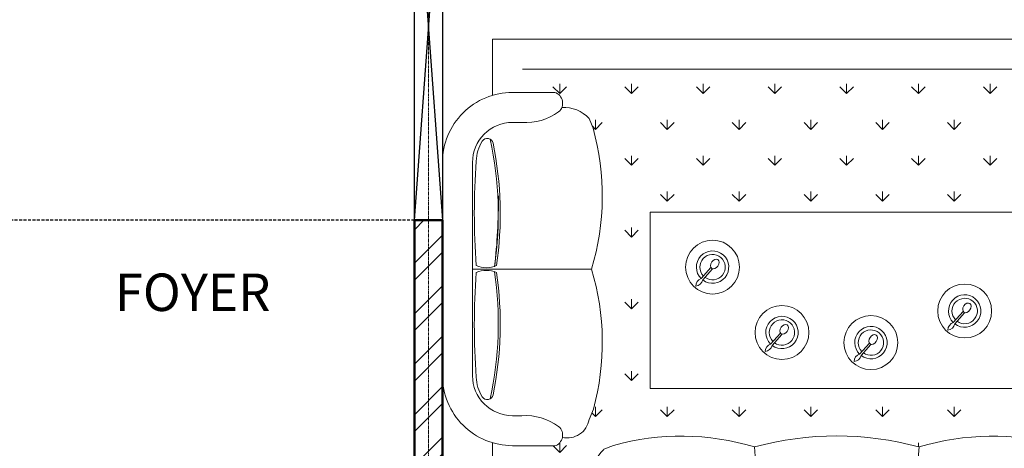
# Model space of a CAD drawing. Units: inches. Extents: x 261 to 2725, y 291 to 1454.
# Tile 10 of 35: x 688 to 898, y 550 to 641. Entities that reach past the tile are written whole.
import ezdxf

# ---------------------------------------------------------------- set-up
doc = ezdxf.new("R2010")
doc.units = ezdxf.units.IN
doc.linetypes.add('CENTER', pattern=[2, 1.25, -0.25, 0.25, -0.25])
doc.linetypes.add('DASHED', pattern=[19.05, 12.7, -6.35])
for name, color, linetype, lineweight in [('A-ANNO-DIMS', 136, 'Continuous', 18), ('A-AREA-IDEN', 18, 'Continuous', 18), ('A-FURN', 30, 'Continuous', 18), ('A-GRID', 251, 'CENTER', 13), ('A-ROOF-PRGL', 25, 'Continuous', 25), ('A-WALL', 222, 'Continuous', 50), ('A-WALL-OVHD', 222, 'DASHED', 25), ('A-WALL-PATT', 243, 'Continuous', 13)]:
    doc.layers.add(name, color=color, linetype=linetype, lineweight=lineweight)
doc.styles.get("Standard").update_dxf_attribs({"font": 'arial.ttf'})
doc.dimstyles.new('ISO-25', dxfattribs={"dimtxt": 12, "dimasz": 6, "dimexe": 1.25, "dimexo": 0.625, "dimtad": 1, "dimdec": 0, "dimlunit": 3, "dimtxsty": 'Standard', "dimblk": 'ARCHTICK', "dimcen": 2.5, "dimadec": 0, "dimazin": 0, "dimtfac": 1, "dimtdec": 0, "dimtmove": 0, "dimatfit": 3, "dimfxl": 1, "dimfxlon": 1, "dimarcsym": 0})

# ---------------------------------------------------------------- blocks, each defined once
blk = doc.blocks.new('A$C29956593')
for p, q in [((1017.8, 2786), (2742.6, 2786)), ((2910.7, 2786), (2742.6, 2786)), ((3602, 2800.7), (3586.8, 2719.3)), ((3630, 2728.1), (3602, 2800.7)), ((3742.2, 2770.6), (3716.5, 2736.8)), ((3730.5, 2659.2), (3742.2, 2770.6)), ((303.3, 2712.1), (296.9, 2710.1)), ((306.1, 2701.8), (303.3, 2712.1)), ((869.5, 2753), (870.7, 2751.8)), ((3447.8, 2749.3), (3463, 2718.1)), ((3486.3, 2729.3), (3447.8, 2749.3)), ((3463, 2718.1), (3488.7, 2658)), ((3547.1, 2656.7), (3486.3, 2729.3)), ((3551.8, 2734.3), (3547.1, 2656.7)), ((3586.8, 2684.2), (3551.8, 2734.3)), ((3586.8, 2719.3), (3589.1, 2643)), ((3644.1, 2670.5), (3630, 2728.1)), ((3716.5, 2736.8), (3682.6, 2663)), ((3811.1, 2721.8), (3772.6, 2710.5)), ((3792.4, 2665.5), (3811.1, 2721.8)), ((113, 2666.3), (113, 2216.3)), ((563, 2666.3), (113, 2666.3)), ((257.1, 2665), (256.2, 2657.4)), ((265.8, 2668.1), (257.1, 2665)), ((259.7, 2679.5), (257.9, 2671.6)), ((257.9, 2671.6), (265.8, 2668.1)), ((269.9, 2678.1), (259.7, 2679.5)), ((268, 2691.2), (264.2, 2685.9)), ((264.2, 2685.9), (269.9, 2678.1)), ((267.7, 2639.4), (270.2, 2671)), ((276.9, 2686.9), (268, 2691.2)), ((270.2, 2671), (283.9, 2691.1)), ((278.2, 2702.6), (273.3, 2697.8)), ((273.3, 2697.8), (276.9, 2686.9)), ((285.5, 2696.3), (278.2, 2702.6)), ((283.9, 2691.1), (302.3, 2697.9)), ((290.3, 2707.8), (284.9, 2706)), ((284.9, 2706), (285.5, 2696.3)), ((296.9, 2700.7), (290.3, 2707.8)), ((296.9, 2710.1), (296.9, 2700.7)), ((302.3, 2697.9), (322.4, 2697.8)), ((309.1, 2711), (306.1, 2701.8)), ((314.8, 2711.2), (309.1, 2711)), ((318.9, 2702.4), (314.8, 2711.2)), ((322.6, 2710.2), (318.9, 2702.4)), ((322.4, 2697.8), (339.2, 2688.6)), ((328.8, 2709.2), (322.6, 2710.2)), ((327.9, 2698.5), (328.8, 2709.2)), ((333.7, 2706), (327.9, 2698.5)), ((338.4, 2703.2), (333.7, 2706)), ((338.4, 2693.8), (338.4, 2703.2)), ((345.6, 2700), (338.4, 2693.8)), ((339.2, 2688.6), (351, 2673.6)), ((351, 2695.6), (345.6, 2700)), ((345.9, 2686.3), (351, 2695.6)), ((355.4, 2689.1), (345.9, 2686.3)), ((351, 2673.6), (355.9, 2654.7)), ((354.8, 2675.8), (359.4, 2683.1)), ((363.7, 2677.8), (354.8, 2675.8)), ((359.4, 2683.1), (355.4, 2689.1)), ((358, 2664.3), (365.7, 2670.6)), ((367.5, 2662.1), (358, 2664.3)), ((365.7, 2670.6), (363.7, 2677.8)), ((563, 2216.3), (563, 2666.3)), ((3395.2, 2706.8), (3416.2, 2674.3)), ((3453.6, 2676.8), (3395.2, 2706.8)), ((3416.2, 2674.3), (3463, 2616.7)), ((3502.7, 2650.5), (3453.6, 2676.8)), ((3682.6, 2663), (3610.3, 2495.9)), ((3635.9, 2584.1), (3644.1, 2670.5)), ((3772.6, 2710.5), (3732.8, 2670.5)), ((3766.7, 2622.9), (3792.4, 2665.5)), ((255.7, 2654.1), (254.5, 2644.2)), ((254.5, 2644.2), (263.6, 2641.2)), ((263.6, 2641.2), (254.7, 2635.1)), ((254.7, 2635.1), (255.8, 2629)), ((265.6, 2653.6), (255.7, 2654.1)), ((255.8, 2629), (265, 2627.7)), ((256.2, 2657.4), (265.6, 2653.6)), ((265, 2627.7), (257.1, 2621.8)), ((257.1, 2621.8), (257.6, 2614.3)), ((257.6, 2614.3), (266.7, 2613.4)), ((266.7, 2613.4), (258.5, 2609)), ((269.6, 2618.4), (267.7, 2639.4)), ((267.7, 2616.4), (269.6, 2618.4)), ((269.4, 2615), (267.7, 2616.4)), ((270.3, 2600.3), (269.4, 2615)), ((345.1, 2616), (342.8, 2608.6)), ((349.3, 2635.7), (345.1, 2629.6)), ((345.1, 2629.6), (348.7, 2623.5)), ((348.7, 2623.5), (345.1, 2616)), ((346.5, 2598), (349, 2613.2)), ((349, 2613.2), (352.7, 2620.7)), ((355.9, 2654.7), (349.3, 2635.7)), ((352.6, 2622.8), (357.2, 2624.6)), ((352.7, 2620.7), (352.6, 2622.8)), ((353.1, 2636.5), (363.4, 2637.8)), ((360.9, 2631.3), (353.1, 2636.5)), ((357.2, 2624.6), (360.9, 2631.3)), ((357.4, 2651), (368.4, 2653.8)), ((366.3, 2646), (357.4, 2651)), ((363.4, 2637.8), (366.3, 2646)), ((368.4, 2653.8), (367.5, 2662.1)), ((2910.7, 2636), (1017.8, 2636)), ((1552.3, 2040.1), (1598.4, 2636)), ((2376.2, 2040.1), (2336.4, 2636)), ((3463, 2616.7), (3512, 2567.8)), ((3557.6, 2604.2), (3502.7, 2650.5)), ((3545.9, 2656.7), (3559.9, 2601.7)), ((3589.1, 2643), (3606.7, 2581.6)), ((3686.1, 2581.6), (3730.5, 2659.2)), ((3727.7, 2578), (3766.7, 2622.9)), ((3859, 2620.4), (3783.1, 2611.7)), ((3891.7, 2610.4), (3859, 2620.4)), ((216.6, 2403), (304.3, 2601.6)), ((231.9, 2406.6), (308.2, 2579.2)), ((258.5, 2609), (258.5, 2601.3)), ((258.5, 2601.3), (267.9, 2601.3)), ((267.9, 2601.3), (258.9, 2597.3)), ((258.9, 2597.3), (259.1, 2591.7)), ((259.1, 2591.7), (268.7, 2590.5)), ((268.7, 2590.5), (260.3, 2584.2)), ((260.3, 2584.2), (260.7, 2578.8)), ((260.7, 2578.8), (269.3, 2577.7)), ((261.3, 2572.2), (261.1, 2568.5)), ((261.1, 2568.5), (263.9, 2566.2)), ((269.3, 2577.7), (261.3, 2572.2)), ((263.9, 2566.2), (269, 2563.6)), ((269.2, 2568), (274, 2569.4)), ((272.1, 2566.8), (269.2, 2568)), ((272.6, 2580.5), (270.3, 2600.3)), ((273.1, 2564.2), (272.1, 2566.8)), ((274, 2569.4), (272.6, 2580.5)), ((275.7, 2559.9), (273.1, 2564.2)), ((310.5, 2576.5), (293.3, 2537.7)), ((304.3, 2601.6), (308.5, 2603.2)), ((308.2, 2579.2), (319.2, 2584.7)), ((308.5, 2603.2), (339.5, 2589.5)), ((314.4, 2581.6), (310.5, 2576.5)), ((310.5, 2576.5), (317.7, 2557.8)), ((321.5, 2581.9), (314.4, 2581.6)), ((319.2, 2584.7), (336.1, 2577.2)), ((320.4, 2560.1), (321.5, 2581.9)), ((335.5, 2575.7), (321.5, 2581.9)), ((338.2, 2583.2), (333.9, 2571.3)), ((333.9, 2571.3), (338.3, 2569.4)), ((340.3, 2593.4), (338.2, 2583.2)), ((338.3, 2569.4), (343.5, 2581.9)), ((356, 2566.7), (340.1, 2573.7)), ((342.8, 2608.6), (340.3, 2593.4)), ((340.5, 2551.2), (356, 2566.7)), ((340.7, 2575.2), (360.9, 2566.2)), ((343.5, 2581.9), (346.5, 2598)), ((344.5, 2587.2), (452.3, 2539.6)), ((356, 2566.7), (360.5, 2561.3)), ((360.9, 2566.2), (365, 2555.9)), ((3329.8, 2610.4), (3384.7, 2576.6)), ((3396.4, 2597.9), (3329.8, 2610.4)), ((3384.7, 2576.6), (3448.9, 2544.1)), ((3454.8, 2577.9), (3396.4, 2597.9)), ((3545.4, 2546.5), (3454.8, 2577.9)), ((3512, 2567.8), (3561.1, 2536.6)), ((3610.3, 2495.9), (3557.6, 2604.2)), ((3606.7, 2581.6), (3610.3, 2495.9)), ((3610.3, 2495.9), (3635.9, 2584.1)), ((3610.3, 2495.9), (3686.1, 2581.6)), ((3704.8, 2564.1), (3610.3, 2495.9)), ((3783.1, 2611.7), (3704.8, 2564.1)), ((3786.6, 2540.3), (3828.6, 2579.1)), ((3828.6, 2579.1), (3891.7, 2610.4)), ((269, 2563.6), (270.6, 2556.3)), ((270.6, 2556.3), (273.2, 2552.7)), ((273.2, 2552.7), (280.8, 2548.3)), ((277.9, 2556.2), (275.7, 2559.9)), ((282.7, 2552.6), (277.9, 2556.2)), ((283.4, 2480.1), (317.7, 2557.8)), ((365, 2555.9), (288, 2381.8)), ((294.1, 2520.1), (291.1, 2509.4)), ((293.3, 2537.7), (293, 2529.2)), ((293, 2529.2), (294.1, 2520.1)), ((306.4, 2470), (340.7, 2547.7)), ((317.7, 2557.8), (320.4, 2560.1)), ((320.4, 2560.1), (340.5, 2551.2)), ((342.2, 2516), (336.2, 2510.1)), ((340.7, 2547.7), (340.5, 2551.2)), ((359.4, 2554.9), (340.7, 2547.7)), ((359.4, 2554.9), (342.2, 2516)), ((360.5, 2561.3), (359.4, 2554.9)), ((453.9, 2535.4), (366.2, 2336.9)), ((378.8, 2560), (375, 2551.4)), ((375, 2551.4), (389.4, 2545)), ((393.2, 2553.7), (378.8, 2560)), ((389.4, 2545), (393.2, 2553.7)), ((399, 2551.1), (395.2, 2542.5)), ((395.2, 2542.5), (409.6, 2536.1)), ((413.4, 2544.8), (399, 2551.1)), ((409.6, 2536.1), (413.4, 2544.8)), ((419.1, 2542.2), (415.3, 2533.6)), ((415.3, 2533.6), (429.7, 2527.2)), ((433.5, 2535.9), (419.1, 2542.2)), ((429.7, 2527.2), (433.5, 2535.9)), ((452.3, 2539.6), (453.9, 2535.4)), ((688, 2553), (563, 2553)), ((3431.3, 2553), (3240.6, 2553)), ((3306.4, 2511.5), (3342.6, 2541.6)), ((3339.1, 2520.3), (3306.4, 2511.5)), ((3412.7, 2494.7), (3339.1, 2520.3)), ((3342.6, 2541.6), (3405.7, 2532.8)), ((3405.7, 2532.8), (3548.9, 2514.2)), ((3448.9, 2544.1), (3610.3, 2495.9)), ((3561.1, 2536.6), (3610.3, 2495.9)), ((3680.3, 2506.5), (3746.9, 2516.5)), ((3746.9, 2516.5), (3786.6, 2540.3)), ((3912.8, 2519), (3797.1, 2546.6)), ((3853.9, 2489.7), (3912.8, 2519)), ((283.4, 2480.1), (254.8, 2415.4)), ((266.8, 2458.2), (272.7, 2467.7)), ((272.7, 2467.7), (279, 2482.1)), ((306.4, 2470), (277.8, 2405.2)), ((291.1, 2509.4), (279, 2482.1)), ((304.3, 2453.7), (310.7, 2468.1)), ((322.8, 2495.4), (310.7, 2468.1)), ((328.7, 2504.8), (322.8, 2495.4)), ((336.2, 2510.1), (328.7, 2504.8)), ((349.4, 2497.4), (353.2, 2506)), ((360.9, 2492.3), (349.4, 2497.4)), ((353.2, 2506), (364.8, 2500.9)), ((355.6, 2456.8), (359.4, 2465.5)), ((359.4, 2465.5), (368, 2461.6)), ((364.8, 2500.9), (360.9, 2492.3)), ((362.6, 2472.7), (366.4, 2481.3)), ((371.2, 2468.8), (362.6, 2472.7)), ((366.4, 2481.3), (375, 2477.5)), ((369.6, 2488.5), (373.4, 2497.1)), ((378.2, 2484.7), (369.6, 2488.5)), ((375, 2477.5), (371.2, 2468.8)), ((373.4, 2497.1), (382, 2493.3)), ((377, 2466.3), (380.8, 2474.9)), ((385.6, 2462.5), (377, 2466.3)), ((382, 2493.3), (378.2, 2484.7)), ((380.8, 2474.9), (389.4, 2471.1)), ((384, 2482.1), (387.8, 2490.7)), ((392.6, 2478.3), (384, 2482.1)), ((389.4, 2471.1), (385.6, 2462.5)), ((387.8, 2490.7), (396.4, 2486.9)), ((391.4, 2459.9), (395.2, 2468.6)), ((396.4, 2486.9), (392.6, 2478.3)), ((395.2, 2468.6), (403.8, 2464.8)), ((398.3, 2475.8), (402.2, 2484.4)), ((407, 2471.9), (398.3, 2475.8)), ((402.2, 2484.4), (410.8, 2480.6)), ((410.8, 2480.6), (407, 2471.9)), ((3306.4, 2461.5), (3338, 2474)), ((3338, 2474), (3388.2, 2495.2)), ((3388.2, 2495.2), (3445.4, 2494)), ((3445.4, 2494), (3517.9, 2492.7)), ((3610.3, 2495.9), (3461.8, 2462.7)), ((3508.5, 2461.5), (3610.3, 2495.9)), ((3517.9, 2492.7), (3610.3, 2495.9)), ((3576.3, 2462.7), (3610.3, 2495.9)), ((3610.3, 2495.9), (3602, 2455.2)), ((3610.3, 2495.9), (3680.3, 2506.5)), ((3610.3, 2495.9), (3651.1, 2485.2)), ((3663.9, 2380.1), (3610.3, 2495.9)), ((3610.3, 2495.9), (3620.7, 2443.9)), ((3665.1, 2452.7), (3610.3, 2495.9)), ((3760.9, 2427.6), (3637.7, 2488.7)), ((3651.1, 2485.2), (3752.7, 2471.5)), ((3702.5, 2499), (3660.1, 2503.8)), ((3781.9, 2481.5), (3702.5, 2499)), ((3731.7, 2512.8), (3846.2, 2496.5)), ((3752.7, 2471.5), (3828.6, 2436.4)), ((3849.7, 2455.2), (3781.9, 2481.5)), ((3846.2, 2496.5), (3871.9, 2474)), ((3871.9, 2474), (3891.7, 2447.7)), ((236.1, 2408.2), (253.3, 2447)), ((253.3, 2447), (259.3, 2452.9)), ((259.3, 2452.9), (266.8, 2458.2)), ((285, 2386.6), (302.2, 2425.4)), ((301.3, 2443), (304.3, 2453.7)), ((302.5, 2433.9), (301.3, 2443)), ((302.2, 2425.4), (302.5, 2433.9)), ((314.6, 2371.8), (338.1, 2425)), ((317.2, 2420.5), (315.3, 2416.2)), ((315.3, 2416.2), (326.8, 2411.1)), ((328.7, 2415.4), (317.2, 2420.5)), ((321, 2429.1), (319.1, 2424.8)), ((319.1, 2424.8), (330.6, 2419.7)), ((332.5, 2424), (321, 2429.1)), ((330.6, 2419.7), (332.5, 2424)), ((338.1, 2425), (379.8, 2406.6)), ((348.6, 2441), (352.4, 2449.6)), ((357.2, 2437.2), (348.6, 2441)), ((352.4, 2449.6), (361, 2445.8)), ((364.2, 2453), (355.6, 2456.8)), ((361, 2445.8), (357.2, 2437.2)), ((363, 2434.6), (366.8, 2443.3)), ((371.6, 2430.8), (363, 2434.6)), ((368, 2461.6), (364.2, 2453)), ((366.8, 2443.3), (375.4, 2439.5)), ((370, 2450.5), (373.8, 2459.1)), ((378.6, 2446.7), (370, 2450.5)), ((375.4, 2439.5), (371.6, 2430.8)), ((373.8, 2459.1), (382.4, 2455.3)), ((377.4, 2428.3), (381.2, 2436.9)), ((386, 2424.5), (377.4, 2428.3)), ((382.4, 2455.3), (378.6, 2446.7)), ((381.2, 2436.9), (389.8, 2433.1)), ((384.4, 2444.1), (388.2, 2452.7)), ((393, 2440.3), (384.4, 2444.1)), ((389.8, 2433.1), (386, 2424.5)), ((388.2, 2452.7), (396.8, 2448.9)), ((400, 2456.1), (391.4, 2459.9)), ((396.8, 2448.9), (393, 2440.3)), ((403.8, 2464.8), (400, 2456.1)), ((667.8, 2436), (667.8, 2224.3)), ((817.8, 2436), (817.8, 2388.1)), ((3110.7, 2388.1), (3110.7, 2436)), ((3260.7, 2436), (3260.7, 2224.3)), ((3321.6, 2453.9), (3306.4, 2461.5)), ((3369.5, 2446.4), (3321.6, 2453.9)), ((3410.4, 2443.9), (3369.5, 2446.4)), ((3376.5, 2402.6), (3433.8, 2435.2)), ((3461.8, 2462.7), (3410.4, 2443.9)), ((3433.8, 2435.2), (3473.5, 2448.9)), ((3526, 2419.4), (3468.8, 2388.9)), ((3473.5, 2448.9), (3508.5, 2461.5)), ((3510.9, 2402.6), (3547.1, 2442.7)), ((3547.1, 2442.7), (3576.3, 2462.7)), ((3602, 2455.2), (3571.6, 2383.8)), ((3583.3, 2373.8), (3596, 2441.2)), ((3620.7, 2443.9), (3609, 2337.5)), ((3637.7, 2436.6), (3704.8, 2385.1)), ((3717.7, 2423.9), (3665.1, 2452.7)), ((3778.4, 2391.4), (3717.7, 2423.9)), ((3831, 2380.1), (3760.9, 2427.6)), ((3828.6, 2436.4), (3904.6, 2381.3)), ((3906.9, 2438.9), (3849.7, 2455.2)), ((3891.7, 2447.7), (3906.9, 2438.9)), ((218.2, 2398.9), (216.6, 2403)), ((362.1, 2335.3), (218.2, 2398.9)), ((236, 2396.2), (231.9, 2406.6)), ((235, 2401.8), (236.1, 2408.2)), ((239.5, 2396.4), (235, 2401.8)), ((279.1, 2377.1), (236, 2396.2)), ((236.1, 2408.2), (254.8, 2415.4)), ((254.9, 2411.9), (239.5, 2396.4)), ((274, 2381.1), (239.5, 2396.4)), ((254.8, 2415.4), (254.9, 2411.9)), ((254.9, 2411.9), (275.1, 2403)), ((275.1, 2403), (274, 2381.1)), ((274, 2381.1), (281, 2381.5)), ((277.8, 2405.2), (275.1, 2403)), ((285, 2386.6), (277.8, 2405.2)), ((288, 2381.8), (279.1, 2377.1)), ((281, 2381.5), (285, 2386.6)), ((301.9, 2386), (300, 2381.7)), ((300, 2381.7), (311.5, 2376.6)), ((313.4, 2380.9), (301.9, 2386)), ((305.7, 2394.6), (303.8, 2390.3)), ((303.8, 2390.3), (315.3, 2385.2)), ((317.3, 2389.5), (305.7, 2394.6)), ((309.6, 2403.2), (307.6, 2398.9)), ((307.6, 2398.9), (319.2, 2393.8)), ((321.1, 2398.1), (309.6, 2403.2)), ((313.4, 2411.9), (311.5, 2407.5)), ((311.5, 2407.5), (323, 2402.5)), ((311.5, 2376.6), (313.4, 2380.9)), ((324.9, 2406.8), (313.4, 2411.9)), ((356.3, 2353.3), (314.6, 2371.8)), ((315.3, 2385.2), (317.3, 2389.5)), ((319.2, 2393.8), (321.1, 2398.1)), ((323, 2402.5), (324.9, 2406.8)), ((326.8, 2411.1), (328.7, 2415.4)), ((379.8, 2406.6), (356.3, 2353.3)), ((667.8, 2403), (563, 2403)), ((3374.8, 2403), (3260.7, 2403)), ((3334.4, 2368.8), (3376.5, 2402.6)), ((3397.5, 2376.3), (3334.4, 2368.8)), ((3374.8, 2403), (3375.8, 2402)), ((3468.8, 2388.9), (3397.5, 2376.3)), ((3444.3, 2326.3), (3492.2, 2378.8)), ((3492.2, 2378.8), (3510.9, 2402.6)), ((3563.4, 2380.1), (3500.4, 2305)), ((3571.6, 2383.8), (3505, 2356.3)), ((3558.8, 2332.5), (3589.6, 2405.9)), ((3581, 2306.2), (3583.3, 2373.8)), ((3617.5, 2415.2), (3640.5, 2363.8)), ((3696.6, 2361.3), (3656.9, 2397.6)), ((3703.6, 2267.4), (3663.9, 2380.1)), ((3704.8, 2385.1), (3766.7, 2347.5)), ((3816.9, 2347.5), (3778.4, 2391.4)), ((3904.6, 2381.3), (3831, 2380.1)), ((366.2, 2336.9), (362.1, 2335.3)), ((3430.2, 2248.7), (3444.3, 2326.3)), ((3505, 2356.3), (3453.6, 2298.7)), ((3500.4, 2305), (3514.4, 2361.3)), ((3514.4, 2259.9), (3558.8, 2332.5)), ((3609, 2337.5), (3611.3, 2274.9)), ((3640.5, 2363.8), (3649.9, 2277.4)), ((3673.6, 2352.7), (3721.2, 2286.2)), ((3772.6, 2305), (3696.6, 2361.3)), ((3766.7, 2347.5), (3812.3, 2318.8)), ((3812.3, 2318.8), (3838, 2295)), ((3838, 2295), (3816.9, 2347.5)), ((3453.6, 2298.7), (3430.2, 2248.7)), ((3581.2, 2312.4), (3540.1, 2262.4)), ((3585.6, 2234.9), (3581, 2306.2)), ((3611.3, 2274.9), (3600.8, 2206.1)), ((3649.9, 2277.4), (3693.1, 2219.9)), ((3721.2, 2286.2), (3800.6, 2259.9)), ((3800.6, 2259.9), (3772.6, 2305)), ((657.5, 2246.7), (623.8, 2213)), ((657.5, 2246.7), (691.1, 2213)), ((657.5, 2246.7), (657.5, 2199.1)), ((3507.4, 2226.1), (3514.4, 2259.9)), ((3521.4, 2204.8), (3507.4, 2226.1)), ((3540.1, 2262.4), (3520.2, 2226.1)), ((3520.2, 2226.1), (3521.4, 2204.8)), ((3595, 2191.1), (3585.6, 2234.9)), ((3687.6, 2019.2), (3687.6, 2227.2)), ((3693.1, 2219.9), (3714.1, 2211.1)), ((3714.1, 2211.1), (3703.6, 2267.4)), ((113, 2216.3), (563, 2216.3)), ((314.4, 2216.3), (314.4, 2031.9)), ((328.6, 2216.3), (331.9, 2213)), ((464.4, 2216.3), (464.4, 2033.7)), ((3600.8, 2206.1), (3595, 2191.1)), ((350, 2033.7), (561.7, 2033.7)), ((477.8, 2067.1), (444.2, 2033.4)), ((477.8, 2067.1), (511.5, 2033.4)), ((477.9, 2067.1), (477.9, 2019.5)), ((798.2, 2052), (847, 2032.1)), ((815.1, 2045.1), (803.4, 2033.4)), ((837.1, 2036.1), (837.1, 2019.5)), ((1555.5, 2039.2), (1555.5, 2019.5)), ((3130.4, 2052), (3081.5, 2032.1)), ((3351.5, 2067.1), (3317.9, 2033.4)), ((3351.5, 2067.1), (3351.5, 2019.5)), ((3351.5, 2067.1), (3383.5, 2035.1)), ((3588.1, 2033.7), (3376.4, 2035.2)), ((350, 1883.7), (397.8, 1883.7)), ((755.2, 1851.4), (733.9, 1903.4)), ((1016.7, 1887.5), (983, 1853.8)), ((1016.7, 1887.5), (1016.7, 1839.9)), ((1016.7, 1887.5), (1050.3, 1853.8)), ((1375.9, 1887.5), (1342.2, 1853.8)), ((1375.9, 1887.5), (1375.9, 1839.9)), ((1375.9, 1887.5), (1409.5, 1853.8)), ((1735.1, 1887.5), (1701.4, 1853.8)), ((1735.1, 1887.5), (1735.1, 1839.9)), ((1735.1, 1887.5), (1768.8, 1853.8)), ((2094.3, 1887.5), (2060.6, 1853.8)), ((2094.3, 1887.5), (2128, 1853.8)), ((2094.3, 1887.5), (2094.3, 1839.9)), ((2453.5, 1887.5), (2419.8, 1853.8)), ((2453.5, 1887.5), (2487.2, 1853.8)), ((2453.5, 1887.5), (2453.5, 1839.9)), ((2812.7, 1887.5), (2779, 1853.8)), ((2812.7, 1887.5), (2812.7, 1839.9)), ((2812.7, 1887.5), (2846.4, 1853.8)), ((3171.9, 1887.5), (3138.2, 1853.8)), ((3171.9, 1887.5), (3171.9, 1839.9)), ((3171.9, 1887.5), (3190.2, 1869.2)), ((3182.9, 1851.4), (3204.2, 1903.4)), ((3588.1, 1883.7), (3540.3, 1883.7)), ((1039.5, 1747.2), (2898.7, 1747.2)), ((1039.5, 864.7), (1039.5, 1747.2)), ((2898.7, 1747.2), (2898.7, 864.7)), ((0, 1683.7), (0, 783.9)), ((150, 615.8), (150, 1683.7)), ((837.1, 1707.9), (803.4, 1674.2)), ((837.1, 1707.9), (870.7, 1674.2)), ((837.1, 1707.9), (837.1, 1660.3)), ((2992.3, 1707.9), (2958.6, 1674.2)), ((2992.3, 1707.9), (2992.3, 1660.3)), ((2992.3, 1707.9), (3026, 1674.2)), ((3788.1, 615.8), (3788.1, 1683.7)), ((3938.1, 1683.7), (3938.1, 783.9)), ((1793.5, 1527.3), (1842.4, 1582.3)), ((1801, 1520.6), (1850, 1575.7)), ((2239, 1476.7), (2287.9, 1531.7)), ((1016.7, 1528.3), (983, 1494.6)), ((1016.7, 1528.3), (1050.3, 1494.6)), ((1016.7, 1528.3), (1016.7, 1480.6)), ((2246.5, 1470), (2295.4, 1525.1)), ((1324, 1369.2), (1372.9, 1424.1)), ((1331.5, 1362.5), (1380.5, 1417.6)), ((837.1, 1348.7), (803.4, 1315)), ((837.1, 1348.7), (870.7, 1315)), ((837.1, 1348.7), (837.1, 1301)), ((2992.3, 1348.7), (2958.6, 1315)), ((2992.3, 1348.7), (2992.3, 1301)), ((2992.3, 1348.7), (3026, 1315)), ((2586.6, 1149.5), (2635.5, 1204.5)), ((2594.1, 1142.8), (2643.1, 1197.9)), ((745.9, 1150.3), (150, 1150.5)), ((1016.7, 1169), (983, 1135.4)), ((1016.7, 1169.1), (1016.7, 1121.4)), ((1016.7, 1169), (1050.3, 1135.4)), ((3192.2, 1150.3), (3788.1, 1150.5)), ((837.1, 989.4), (803.4, 955.8)), ((837.1, 989.5), (837.1, 941.8)), ((837.1, 989.4), (870.7, 955.8)), ((2992.3, 989.4), (2958.6, 955.8)), ((2992.3, 989.5), (2992.3, 941.8)), ((2992.3, 989.4), (3026, 955.8)), ((2898.7, 864.7), (1039.5, 864.7)), ((1016.7, 809.8), (983, 776.2)), ((1016.7, 809.9), (1016.7, 762.2)), ((1016.7, 809.8), (1050.3, 776.2)), ((1375.9, 809.8), (1342.2, 776.2)), ((1375.9, 809.9), (1375.9, 762.2)), ((1375.9, 809.8), (1409.5, 776.2)), ((1735.1, 809.8), (1701.4, 776.2)), ((1735.1, 809.9), (1735.1, 762.2)), ((1735.1, 809.8), (1768.8, 776.2)), ((2094.3, 809.8), (2060.6, 776.2)), ((2094.3, 809.9), (2094.3, 762.2)), ((2094.3, 809.8), (2128, 776.2)), ((2453.5, 809.8), (2419.8, 776.2)), ((2453.5, 809.9), (2453.5, 762.2)), ((2453.5, 809.8), (2487.2, 776.2)), ((2812.7, 809.8), (2779, 776.2)), ((2812.7, 809.9), (2812.7, 762.2)), ((2812.7, 809.8), (2846.4, 776.2)), ((0, 783.9), (0, 615.8)), ((3938.1, 783.9), (3938.1, 615.8)), ((837.1, 630.2), (803.4, 596.6)), ((837.1, 630.2), (837.1, 582.6)), ((837.1, 630.2), (870.7, 596.6)), ((1196.3, 630.2), (1162.6, 596.6)), ((1196.3, 630.2), (1196.3, 582.6)), ((1196.3, 630.2), (1229.9, 596.6)), ((1555.5, 630.2), (1521.8, 596.6)), ((1555.5, 630.2), (1555.5, 582.6)), ((1555.5, 630.2), (1589.2, 596.6)), ((1914.7, 630.2), (1881, 596.6)), ((1914.7, 630.2), (1914.7, 582.6)), ((1914.7, 630.2), (1948.4, 596.6)), ((2273.9, 630.2), (2240.2, 596.6)), ((2273.9, 630.2), (2273.9, 582.6)), ((2273.9, 630.2), (2307.6, 596.6)), ((2633.1, 630.2), (2599.4, 596.6)), ((2633.1, 630.2), (2633.1, 582.6)), ((2633.1, 630.2), (2666.8, 596.6)), ((2992.3, 630.2), (2958.6, 596.6)), ((2992.3, 630.2), (2992.3, 582.6)), ((2992.3, 630.2), (3026, 596.6)), ((733.9, 396.1), (753.9, 445)), ((1016.7, 450.6), (983, 417)), ((1016.7, 450.6), (1016.7, 403)), ((1016.7, 450.6), (1050.3, 417)), ((1375.9, 450.6), (1342.2, 417)), ((1375.9, 450.6), (1375.9, 403)), ((1375.9, 450.6), (1409.5, 417)), ((1735.1, 450.6), (1701.4, 417)), ((1735.1, 450.6), (1768.8, 417)), ((1735.1, 450.6), (1735.1, 403)), ((2094.3, 450.6), (2060.6, 417)), ((2094.3, 450.6), (2128, 417)), ((2094.3, 450.6), (2094.3, 403)), ((2453.5, 450.6), (2419.8, 417)), ((2453.5, 450.6), (2487.2, 417)), ((2453.5, 450.6), (2453.5, 403)), ((2812.7, 450.6), (2779, 417)), ((2812.7, 450.6), (2846.4, 417)), ((2812.7, 450.6), (2812.7, 403)), ((3171.9, 450.6), (3138.2, 417)), ((3171.9, 450.6), (3188.8, 433.8)), ((3171.9, 450.6), (3171.9, 403)), ((3204.2, 396.1), (3184.2, 445)), ((397.8, 415.8), (350, 415.8)), ((3540.3, 415.8), (3588.1, 415.8)), ((314.4, 267.6), (314.4, 0)), ((350, 265.8), (561.7, 265.8)), ((464.4, 265.8), (464.4, 150)), ((472.6, 265.8), (464.4, 257.6)), ((477.8, 271), (472.6, 265.8)), ((477.8, 271), (483.1, 265.8)), ((477.9, 271), (477.9, 265.8)), ((477.9, 265.8), (477.9, 223.4)), ((483.1, 265.8), (511.5, 237.3)), ((837.1, 271), (803.4, 237.3)), ((837.1, 271), (870.7, 237.3)), ((837.1, 271), (837.1, 223.4)), ((1196.3, 271), (1162.6, 237.3)), ((1196.3, 271), (1196.3, 223.4)), ((1196.3, 271), (1229.9, 237.3)), ((1555.5, 271), (1521.8, 237.3)), ((1555.5, 271), (1555.5, 223.4)), ((1555.5, 271), (1589.2, 237.3)), ((1914.7, 271), (1881, 237.3)), ((1914.7, 271), (1914.7, 223.4)), ((1914.7, 271), (1948.4, 237.3)), ((2273.9, 271), (2240.2, 237.3)), ((2273.9, 271), (2273.9, 223.4)), ((2273.9, 271), (2307.6, 237.3)), ((2633.1, 271), (2599.4, 237.3)), ((2633.1, 271), (2633.1, 223.4)), ((2633.1, 271), (2666.8, 237.3)), ((2992.3, 271), (2958.6, 237.3)), ((2992.3, 271), (2992.3, 223.4)), ((2992.3, 271), (3026, 237.3)), ((3351.5, 271), (3317.9, 237.3)), ((3351.5, 271), (3351.5, 223.4)), ((3351.5, 271), (3385.2, 237.3)), ((3588.1, 265.8), (3376.4, 265.8)), ((3687.6, 0), (3687.6, 280.2)), ((464.4, 150), (3537.6, 150)), ((314.4, 0), (3687.6, 0))]:
    blk.add_line(p, q)
for centre in [(1793, 1517.9), (2238.5, 1467.3), (1323.5, 1359.8), (2586.1, 1140.1)]:
    blk.add_circle(centre, 134.9)
for centre, radius, start, end in [((1017.8, 2436), 350, 90, 180), ((2910.7, 2436), 350, 0, 90), ((1017.8, 2436), 200, 90, 180), ((1011.2, 2436.9), 180, 90, 123.4988), ((1272.9, -801.2), 3428.1, 85.6218, 94.3782), ((1415.2, 2566.2), 129.8, 336.9832, 23.0167), ((1748.3, 2436.9), 180, 90, 123.4988), ((2010, -801.2), 3428.1, 85.6218, 94.3782), ((2152.3, 2566.2), 129.8, 336.9832, 23.0167), ((2513.3, 2566.2), 129.8, 156.9833, 203.0168), ((2655.6, -801.2), 3428.1, 85.6218, 94.3782), ((2910.7, 2436), 200, 0, 90), ((2917.3, 2436.9), 180, 56.5012, 90), ((928.5, 2562), 30, 123.4988, 258.5347), ((1665.5, 2562), 30, 123.4988, 258.5347), ((3000.1, 2562), 30, 281.4653, 56.5012), ((1278, 4285.1), 1778.2, 257.8102, 278.4302), ((1278, 4285.1), 1788.2, 258.5347, 278.2533), ((2015, 4285.1), 1778.2, 257.8102, 278.4302), ((2015, 4285.1), 1788.2, 258.5347, 278.2533), ((2735.9, 5677.7), 3171.8, 263.6902, 270.1225), ((2650.6, 4285.1), 1778.2, 261.5698, 282.1898), ((2650.6, 4285.1), 1788.2, 261.7467, 281.4653), ((534.8, 2371.7), 283.5, 323.9008, 3.3226), ((3381.1, 2366.2), 271.2, 175.359, 216.5496), ((720.5, 2241.3), 56.8, 197.4727, 319.7773), ((3206.5, 2241.3), 56.8, 220.2227, 342.5272), ((918.2, 2179.8), 175.3, 177.1066, 226.7866), ((3010.4, 2179.8), 175.3, 313.2134, 2.8934), ((350, 1683.7), 350, 90, 180), ((544.6, 1981), 56.8, 310.2227, 72.5273), ((1184.5, 3255.7), 1269.7, 254.7297, 286.7871), ((1964.3, 3548.9), 1564, 254.7283, 285.2717), ((2742.7, 3254.2), 1268.2, 253.2031, 285.5373), ((3393.5, 1981), 56.8, 107.4727, 229.7773), ((3588.1, 1683.7), 350, 360, 90), ((624.3, 1883.4), 111.5, 10.3315, 102.4252), ((3313.8, 1883.4), 111.5, 77.5748, 169.6685), ((414.3, 2166.7), 283.5, 266.6774, 306.0992), ((3523.8, 2166.7), 283.5, 233.9008, 273.3226), ((350, 1683.7), 200, 90, 180), ((3588.1, 1683.7), 200, 360, 90), ((-469.7, 1517), 1269.7, 343.2129, 15.2703), ((4407.8, 1517), 1269.7, 164.7297, 196.7871), ((349.1, 1690.3), 180, 146.5012, 180), ((224, 1773), 30, 11.4653, 146.5012), ((-1499.2, 1423.6), 1778.2, 351.5698, 12.1898), ((-1499.2, 1423.6), 1788.2, 351.7467, 11.4653), ((5437.3, 1423.6), 1788.2, 168.5347, 188.2533), ((5437.3, 1423.6), 1778.2, 167.8102, 188.4302), ((3714.1, 1773), 30, 33.4988, 168.5347), ((3589, 1690.3), 180, 360, 33.4988), ((3587.2, 1428.6), 3428.1, 175.6218, 184.3782), ((350.9, 1428.6), 3428.1, 355.6218, 4.3782), ((1793, 1517.9), 81.1, 52.4982, 45.4047), ((1793, 1517.9), 63.6, 53.6389, 44.5926), ((1880.7, 1574), 39.2, 95.4915, 167.8668), ((1837.8, 1612.8), 39.2, 287.9204, 0.3094), ((2238.5, 1467.3), 81.1, 52.4982, 45.4047), ((2238.5, 1467.3), 63.6, 53.6389, 44.5926), ((2326.2, 1523.4), 39.2, 95.4915, 167.8668), ((2283.2, 1562.3), 39.2, 287.9204, 0.3094), ((1323.5, 1359.8), 81.1, 52.4982, 45.4047), ((1411.3, 1415.9), 39.2, 95.4915, 167.8668), ((1368.3, 1454.7), 39.2, 287.9204, 0.3094), ((1323.5, 1359.8), 63.6, 53.6389, 44.5926), ((2673.8, 1196.2), 39.2, 95.4915, 167.8668), ((2630.9, 1235.1), 39.2, 287.9204, 0.3094), ((2586.1, 1140.1), 81.1, 52.4982, 45.4047), ((2586.1, 1140.1), 63.6, 53.6389, 44.5926), ((219.8, 1286.3), 129.8, 246.9833, 293.0168), ((219.8, 1013.2), 129.8, 66.9832, 113.0167), ((-1499.2, 875.9), 1778.2, 347.8102, 8.4302), ((-2891.8, 790.6), 3171.8, 359.8775, 6.3098), ((-468.2, 783.8), 1268.2, 344.4627, 16.7969), ((4406.3, 783.8), 1268.2, 163.2031, 195.5373), ((6829.9, 790.6), 3171.8, 173.6902, 180.1225), ((5437.3, 875.9), 1778.2, 171.5698, 192.1898), ((3718.3, 1286.3), 129.8, 246.9832, 293.0167), ((3718.3, 1013.2), 129.8, 66.9833, 113.0168), ((3587.2, 870.9), 3428.1, 175.6218, 184.3782), ((-1499.2, 875.9), 1788.2, 348.5347, 8.2533), ((5437.3, 875.9), 1788.2, 171.7467, 191.4653), ((350.9, 870.9), 3428.1, 355.6218, 4.3782), ((350, 615.8), 350, 180, 270), ((350, 615.8), 200, 180, 270), ((349.1, 609.2), 180, 180, 213.4988), ((3588.1, 615.8), 200, 270, 0), ((3588.1, 615.8), 350, 270, 0), ((3589, 609.2), 180, 326.5012, 0), ((224, 526.4), 30, 213.4988, 348.5347), ((3714.1, 526.4), 30, 191.4653, 326.5012), ((419.8, 145.5), 271.2, 53.4504, 94.641), ((606.2, 516.1), 175.3, 267.1066, 316.7866), ((3331.9, 516.1), 175.3, 223.2134, 272.8934), ((3518.3, 145.5), 271.2, 85.359, 126.5496), ((544.6, 320), 56.8, 287.4728, 49.7773), ((3393.5, 320), 56.8, 130.2227, 252.5272)]:
    blk.add_arc(centre, radius, start, end)
for centre in [(1781.9, 1502.2), (2227.3, 1451.6), (1312.4, 1344.1), (2575, 1124.5)]:
    blk.add_ellipse(centre, major_axis=(-14.8, -22.2), ratio=0.68685)
blk = doc.blocks.new('_ArchTick')
at = {"color": 0, "linetype": 'ByBlock', "const_width": 0.15}
blk.add_lwpolyline([(-0.5, -0.5), (0.5, 0.5)], dxfattribs=at)
blk = doc.blocks.new('*D86')
at = {"layer": 'A-ANNO-DIMS', "color": 0, "lineweight": -2, "ltscale": 0.07, "transparency": 16777216}
for p, q in [((676.45, 1437.76), (676.45, 1440.01)), ((676.45, 1438.76), (772.45, 1438.76)), ((772.45, 1437.76), (772.45, 1440.01))]:
    blk.add_line(p, q, dxfattribs=at)
at = {"layer": 'Defpoints', "color": 0, "ltscale": 0.07, "transparency": 16777216}
for p in [(772.45, 1438.76), (676.45, 517.47), (772.45, 517.47)]:
    blk.add_point(p, dxfattribs=at)
at = {"layer": 'A-ANNO-DIMS', "color": 0, "lineweight": -2, "ltscale": 0.07, "transparency": 16777216, "xscale": 6, "yscale": 6, "zscale": 6, "rotation": 180}
blk.add_blockref('_ArchTick', (676.45, 1438.76), dxfattribs=at)
at = {"layer": 'A-ANNO-DIMS', "color": 0, "lineweight": -2, "ltscale": 0.07, "transparency": 16777216, "xscale": 6, "yscale": 6, "zscale": 6}
blk.add_blockref('_ArchTick', (772.45, 1438.76), dxfattribs=at)
at = {"layer": 'A-ANNO-DIMS', "color": 0, "ltscale": 0.07, "transparency": 16777216, "insert": (724.45, 1445.51), "char_height": 12, "attachment_point": 5}
blk.add_mtext('8\'-0"', dxfattribs=at)
blk = doc.blocks.new('*D99')
at = {"layer": 'A-ANNO-DIMS', "color": 0, "lineweight": -2, "ltscale": 0.07, "transparency": 16777216}
for p, q in [((825.95, 305.22), (825.95, 302.97)), ((836.95, 305.22), (836.95, 302.97)), ((825.95, 304.22), (836.95, 304.22)), ((836.95, 304.22), (885.42, 304.22))]:
    blk.add_line(p, q, dxfattribs=at)
at = {"layer": 'Defpoints', "color": 0, "ltscale": 0.07, "transparency": 16777216}
for p in [(825.95, 679.47), (836.95, 679.47), (836.95, 304.22)]:
    blk.add_point(p, dxfattribs=at)
at = {"layer": 'A-ANNO-DIMS', "color": 0, "lineweight": -2, "ltscale": 0.07, "transparency": 16777216, "xscale": 6, "yscale": 6, "zscale": 6, "rotation": 180}
blk.add_blockref('_ArchTick', (825.95, 304.22), dxfattribs=at)
at = {"layer": 'A-ANNO-DIMS', "color": 0, "lineweight": -2, "ltscale": 0.07, "transparency": 16777216, "xscale": 6, "yscale": 6, "zscale": 6}
blk.add_blockref('_ArchTick', (836.95, 304.22), dxfattribs=at)
at = {"layer": 'A-ANNO-DIMS', "color": 0, "ltscale": 0.07, "transparency": 16777216, "insert": (864.19, 310.97), "char_height": 12, "attachment_point": 5}
blk.add_mtext('0\'-11"', dxfattribs=at)
blk = doc.blocks.new('*D103')
at = {"layer": 'A-ANNO-DIMS', "color": 0, "lineweight": -2, "ltscale": 0.07, "transparency": 16777216}
for p, q in [((287.06, 1231.47), (284.81, 1231.47)), ((286.06, 439.47), (286.06, 1231.47)), ((287.06, 439.47), (284.81, 439.47))]:
    blk.add_line(p, q, dxfattribs=at)
at = {"layer": 'Defpoints', "color": 0, "ltscale": 0.07, "transparency": 16777216}
for p in [(286.06, 1231.47), (1243.08, 1231.47), (1243.08, 439.47)]:
    blk.add_point(p, dxfattribs=at)
at = {"layer": 'A-ANNO-DIMS', "color": 0, "lineweight": -2, "ltscale": 0.07, "transparency": 16777216, "xscale": 6, "yscale": 6, "zscale": 6}
for p, rotation in [((286.06, 1231.47), 90), ((286.06, 439.47), 270)]:
    blk.add_blockref('_ArchTick', p, dxfattribs=dict(at, rotation=rotation))
at = {"layer": 'A-ANNO-DIMS', "color": 0, "ltscale": 0.07, "transparency": 16777216, "insert": (279.3, 835.47), "char_height": 12, "attachment_point": 5, "rotation": 90}
blk.add_mtext('66\'-0"', dxfattribs=at)
blk = doc.blocks.new('*D107')
at = {"layer": 'A-ANNO-DIMS', "color": 0, "lineweight": -2, "ltscale": 0.07, "transparency": 16777216}
for p, q in [((287.06, 673.47), (284.81, 673.47)), ((286.06, 496.47), (286.06, 673.47)), ((287.06, 496.47), (284.81, 496.47))]:
    blk.add_line(p, q, dxfattribs=at)
at = {"layer": 'Defpoints', "color": 0, "ltscale": 0.07, "transparency": 16777216}
for p in [(286.06, 673.47), (1252.08, 673.47), (1252.08, 496.47)]:
    blk.add_point(p, dxfattribs=at)
at = {"layer": 'A-ANNO-DIMS', "color": 0, "lineweight": -2, "ltscale": 0.07, "transparency": 16777216, "xscale": 6, "yscale": 6, "zscale": 6}
for p, rotation in [((286.06, 673.47), 90), ((286.06, 496.47), 270)]:
    blk.add_blockref('_ArchTick', p, dxfattribs=dict(at, rotation=rotation))
at = {"layer": 'A-ANNO-DIMS', "color": 0, "ltscale": 0.07, "transparency": 16777216, "insert": (279.3, 584.97), "char_height": 12, "attachment_point": 5, "rotation": 90}
blk.add_mtext('14\'-9"', dxfattribs=at)
blk = doc.blocks.new('*D123')
at = {"layer": 'A-ANNO-DIMS', "color": 0, "lineweight": -2, "ltscale": 0.07, "transparency": 16777216}
for p, q in [((287.06, 1054.85), (284.81, 1054.85)), ((286.06, 439.47), (286.06, 1054.85)), ((287.06, 439.47), (284.81, 439.47))]:
    blk.add_line(p, q, dxfattribs=at)
at = {"layer": 'Defpoints', "color": 0, "ltscale": 0.07, "transparency": 16777216}
for p in [(286.06, 1054.85), (2007.71, 1054.85), (2007.71, 439.47)]:
    blk.add_point(p, dxfattribs=at)
at = {"layer": 'A-ANNO-DIMS', "color": 0, "lineweight": -2, "ltscale": 0.07, "transparency": 16777216, "xscale": 6, "yscale": 6, "zscale": 6}
for p, rotation in [((286.06, 1054.85), 90), ((286.06, 439.47), 270)]:
    blk.add_blockref('_ArchTick', p, dxfattribs=dict(at, rotation=rotation))
at = {"layer": 'A-ANNO-DIMS', "color": 0, "ltscale": 0.07, "transparency": 16777216, "insert": (279.22, 747.16), "char_height": 12, "attachment_point": 5, "rotation": 90}
blk.add_mtext('51\'-3 1/2"', dxfattribs=at)

msp = doc.modelspace()

# ---------------------------------------------------------------- hatches: boundary and pattern name
at = {"layer": 'A-WALL-PATT'}
h = msp.add_hatch(dxfattribs=at)
h.set_pattern_fill('ANSI32', color=256, scale=0.8)
h.paths.add_polyline_path([(478.45, 685.47), (580.45, 685.47), (580.45, 691.47), (577.45, 691.47), (577.45, 694.47), (571.45, 694.47), (571.45, 691.47), (478.45, 691.47), (478.45, 721.47), (469.45, 721.47), (469.45, 508.47), (538.45, 508.47), (538.45, 517.47), (478.45, 517.47)])
h.paths.add_polyline_path([(694.45, 517.47), (676.45, 517.47), (676.45, 646.47), (670.45, 646.47), (670.45, 517.47), (610.45, 517.47), (610.45, 508.47), (694.45, 508.47)])
h.paths.add_polyline_path([(676.45, 784.47), (478.45, 784.47), (478.45, 844.47), (469.45, 844.47), (469.45, 745.47), (478.45, 745.47), (478.45, 775.47), (571.45, 775.47), (571.45, 724.47), (577.45, 724.47), (577.45, 775.47), (670.45, 775.47), (670.45, 691.47), (610.45, 691.47), (610.45, 685.47), (670.45, 685.47), (670.45, 682.47), (676.45, 682.47)])
h.paths.add_polyline_path([(955.45, 880.47), (946.45, 880.47), (946.45, 808.47), (778.45, 808.47), (778.45, 799.47), (946.45, 799.47), (946.45, 517.47), (898.45, 517.47), (898.45, 508.47), (955.45, 508.47)])
h.paths.add_polyline_path([(778.45, 598.47), (772.45, 598.47), (772.45, 517.47), (754.45, 517.47), (754.45, 508.47), (826.45, 508.47), (826.45, 517.47), (778.45, 517.47)])
h.paths.add_polyline_path([(955.45, 1090.47), (946.45, 1090.47), (946.45, 1030.47), (817.45, 1030.47), (817.45, 1024.47), (946.45, 1024.47), (946.45, 952.47), (955.45, 952.47)])
h.paths.add_polyline_path([(955.45, 1231.47), (730.45, 1231.47), (730.45, 1222.47), (772.45, 1222.47), (772.45, 1096.47), (766.45, 1096.47), (766.45, 1090.47), (772.45, 1090.47), (772.45, 1006.47), (712.45, 1006.47), (712.45, 1000.47), (778.45, 1000.47), (778.45, 1024.47), (781.45, 1024.47), (781.45, 1030.47), (778.45, 1030.47), (778.45, 1222.47), (946.45, 1222.47), (946.45, 1162.47), (955.45, 1162.47)])
h.paths.add_polyline_path([(694.45, 1231.47), (619.45, 1231.47), (619.45, 1222.47), (646.45, 1222.47), (646.45, 1039.47), (652.45, 1039.47), (652.45, 1090.47), (736.45, 1090.47), (736.45, 1096.47), (652.45, 1096.47), (652.45, 1222.47), (694.45, 1222.47)])
h.paths.add_polyline_path([(571.45, 1231.47), (469.45, 1231.47), (469.45, 1099.47), (478.45, 1099.47), (478.45, 1144.47), (544.45, 1144.47), (544.45, 1153.47), (538.45, 1153.47), (538.45, 1150.47), (478.45, 1150.47), (478.45, 1222.47), (538.45, 1222.47), (538.45, 1183.47), (544.45, 1183.47), (544.45, 1222.47), (571.45, 1222.47)])
h.paths.add_polyline_path([(538.45, 1006.47), (478.45, 1006.47), (478.45, 1051.47), (469.45, 1051.47), (469.45, 940.47), (478.45, 940.47), (478.45, 1000.47), (538.45, 1000.47)])
h.paths.add_polyline_path([(652.45, 1006.47), (652.45, 1009.47), (646.45, 1009.47), (646.45, 1006.47), (586.45, 1006.47), (586.45, 1000.47), (652.45, 1000.47)])
h.paths.add_polyline_path([(1288.08, 973.47), (1243.08, 973.47), (1243.08, 920.97), (1252.08, 920.97), (1252.08, 964.47), (1288.08, 964.47)], flags=17)
h.paths.add_polyline_path([(1402.08, 805.47), (1252.08, 805.47), (1252.08, 848.97), (1243.08, 848.97), (1243.08, 757.47), (1252.08, 757.47), (1252.08, 799.47), (1294.08, 799.47), (1372.08, 799.47), (1372.08, 779.47), (1372.08, 715.47), (1378.08, 715.47), (1378.08, 799.47), (1402.08, 799.47)])
h.paths.add_polyline_path([(1252.08, 721.47), (1243.08, 721.47), (1243.08, 439.47), (1729.08, 439.47), (1729.08, 709.47), (1720.08, 709.47), (1720.08, 679.47), (1582.08, 679.47), (1582.08, 670.47), (1588.08, 670.47), (1588.08, 673.47), (1720.08, 673.47), (1720.08, 559.47), (1690.08, 559.47), (1690.08, 550.47), (1720.08, 550.47), (1720.08, 448.47), (1252.08, 448.47), (1252.08, 496.47), (1312.08, 496.47), (1312.08, 505.47), (1252.08, 505.47), (1252.08, 673.47), (1405.08, 673.47), (1405.08, 679.47), (1378.08, 679.47), (1378.08, 685.47), (1372.08, 685.47), (1372.08, 679.47), (1252.08, 679.47)])
h.paths.add_polyline_path([(1450.08, 550.47), (1480.08, 550.47), (1480.08, 559.47), (1450.08, 559.47), (1450.08, 679.47), (1441.08, 679.47), (1441.08, 673.47), (1444.08, 673.47), (1444.08, 505.47), (1384.08, 505.47), (1384.08, 496.47), (1450.08, 496.47)], flags=17)
h.paths.add_polyline_path([(1618.08, 559.47), (1588.08, 559.47), (1588.08, 634.47), (1582.08, 634.47), (1582.08, 559.47), (1552.08, 559.47), (1552.08, 550.47), (1618.08, 550.47)], flags=17)
h.paths.add_polyline_path([(1564.08, 964.47), (1630.08, 964.47), (1630.08, 973.47), (1477.08, 973.47), (1477.08, 964.47), (1558.08, 964.47), (1558.08, 926.22), (1558.08, 887.97), (1486.08, 887.97), (1486.08, 881.97), (1558.08, 881.97), (1558.08, 805.47), (1450.08, 805.47), (1450.08, 845.97), (1444.08, 845.97), (1444.08, 805.47), (1438.08, 805.47), (1438.08, 799.47), (1564.08, 799.47)], flags=17)
h.paths.add_polyline_path([(1453.08, 973.47), (1408.08, 973.47), (1408.08, 964.47), (1444.08, 964.47), (1444.08, 881.97), (1450.08, 881.97), (1456.08, 881.97), (1456.08, 887.97), (1450.08, 887.97), (1450.08, 964.47), (1453.08, 964.47)], flags=17)
h.paths.add_polyline_path([(1729.08, 1231.47), (1243.08, 1231.47), (1243.08, 1167.47), (1252.08, 1167.47), (1252.08, 1222.47), (1441.08, 1222.47), (1441.08, 1045.47), (1648.08, 1045.47), (1648.08, 1051.47), (1450.08, 1051.47), (1450.08, 1074.47), (1450.08, 1222.47), (1472.08, 1222.47), (1720.08, 1222.47), (1720.08, 1051.47), (1708.08, 1051.47), (1708.08, 1045.47), (1720.08, 1045.47), (1720.08, 973.47), (1702.08, 973.47), (1702.08, 964.47), (1720.08, 964.47), (1720.08, 769.47), (1729.08, 769.47)])
h.paths.add_polyline_path([(2493.71, 1054.85), (2007.71, 1054.85), (2007.71, 439.47), (2214.67, 439.47), (2214.67, 496.47), (2493.71, 496.47)])
h.paths.add_polyline_path([(2016.71, 1045.85), (2304.71, 1045.85), (2304.71, 841.47), (2310.71, 841.47), (2310.71, 1045.85), (2484.71, 1045.85), (2484.71, 805.47), (2310.71, 805.47), (2310.71, 811.47), (2304.71, 811.47), (2304.71, 799.47), (2484.71, 799.47), (2484.71, 679.47), (2304.71, 679.47), (2304.71, 673.47), (2484.71, 673.47), (2484.71, 505.47), (2208.67, 505.47), (2208.67, 448.47), (2016.71, 448.47), (2016.71, 799.47), (2304.71, 799.47), (2304.71, 805.47), (2016.71, 805.47)], flags=16)

# ---------------------------------------------------------------- linework, layer by layer
at = {"layer": 'A-GRID', "ltscale": 0.5}
msp.add_line((775.45, 1330.47), (775.45, 416.47), dxfattribs=at)
at = {"layer": 'A-ROOF-PRGL'}
for p, q in [((772.45, 598.47), (778.45, 679.47)), ((772.45, 679.47), (778.45, 598.47))]:
    msp.add_line(p, q, dxfattribs=at)
msp.add_lwpolyline([(772.45, 679.47), (778.45, 679.47), (778.45, 598.47), (772.45, 598.47)], close=True, dxfattribs=at)
at = {"layer": 'A-WALL'}
for p, q in [((772.45, 517.47), (772.45, 598.47)), ((772.45, 598.47), (778.45, 598.47)), ((778.45, 517.47), (778.45, 598.47))]:
    msp.add_line(p, q, dxfattribs=at)
at = {"layer": 'A-WALL-OVHD', "ltscale": 0.05}
msp.add_line((772.45, 598.47), (676.45, 598.47), dxfattribs=at)

# ---------------------------------------------------------------- block references
at = {"layer": 'A-FURN', "xscale": 0.0426601237233356, "yscale": 0.0426601237233356, "zscale": 0.0426601237233356, "rotation": 180}
msp.add_blockref('A$C29956593', (946.45, 637.08), dxfattribs=at)

# ---------------------------------------------------------------- texts
at = {"layer": 'A-AREA-IDEN', "insert": (704.12, 587.07), "char_height": 8, "attachment_point": 1}
msp.add_mtext_dynamic_manual_height_columns('\\pxqc;{\\fTimes New Roman|b0|i0|c0|p18;FOYER}', width=41.8749, gutter_width=12.5, heights=[0], dxfattribs=at)

# ---------------------------------------------------------------- dimensions: what is measured, and where the dimension line sits
at = {"layer": 'A-ANNO-DIMS', "ltscale": 0.07}
for base, p1, p2, picture, middle in [((772.45, 1438.76), (676.45, 517.47), (772.45, 517.47), '*D86', (724.45, 1445.51)), ((836.95, 304.22), (825.95, 679.47), (836.95, 679.47), '*D99', (864.19, 310.97))]:
    dim = msp.add_linear_dim(base=base, p1=p1, p2=p2, dimstyle='ISO-25', override={"dimdec": 1, "dimlfac": 1, "dimrnd": 0, "dimzin": 1, "dimdsep": 46, "dimlunit": 4, "dimfrac": 2}, dxfattribs=at)
    dim.commit()
    dim.dimension.update_dxf_attribs({"geometry": picture, "text_midpoint": middle})
for base, p1, p2, picture, middle in [((286.06, 1231.47), (1243.08, 439.47), (1243.08, 1231.47), '*D103', (279.3, 835.47)), ((286.06, 1054.85), (2007.71, 439.47), (2007.71, 1054.85), '*D123', (279.22, 747.16)), ((286.06, 673.47), (1252.08, 496.47), (1252.08, 673.47), '*D107', (279.3, 584.97))]:
    dim = msp.add_linear_dim(base=base, p1=p1, p2=p2, angle=90, dimstyle='ISO-25', override={"dimdec": 1, "dimlfac": 1, "dimrnd": 0, "dimzin": 1, "dimdsep": 46, "dimlunit": 4, "dimfrac": 2}, dxfattribs=at)
    dim.commit()
    dim.dimension.update_dxf_attribs({"geometry": picture, "text_midpoint": middle})

doc.saveas('drawing.dxf')
